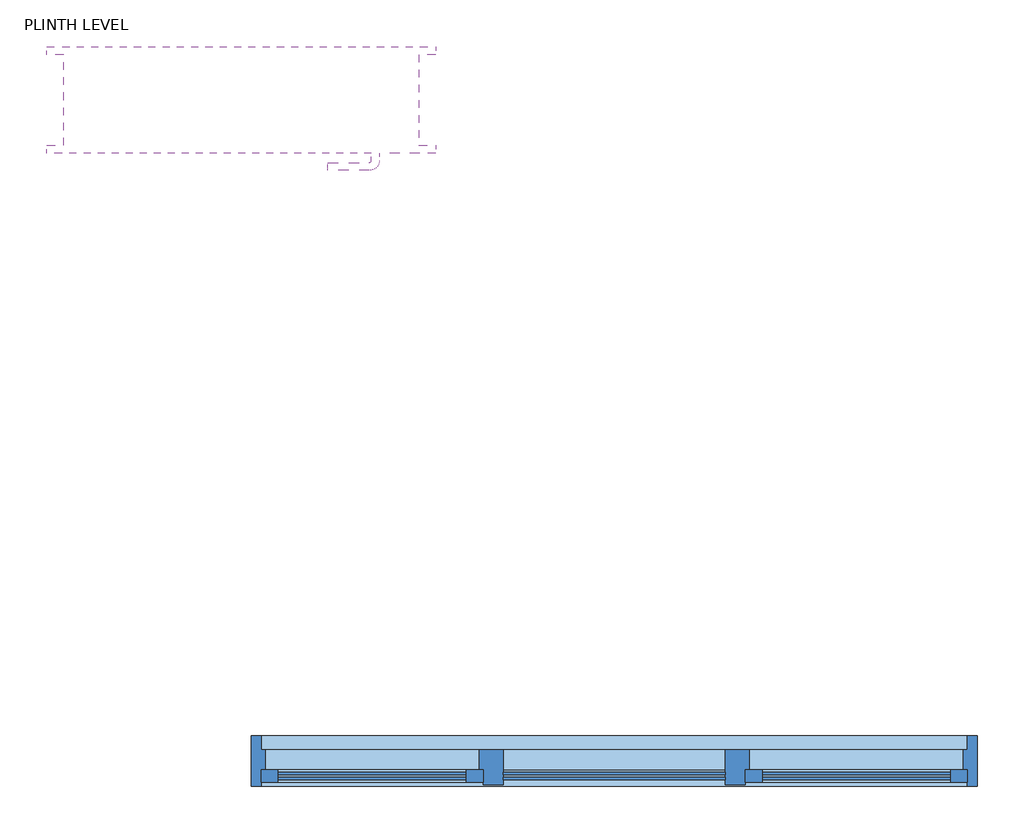
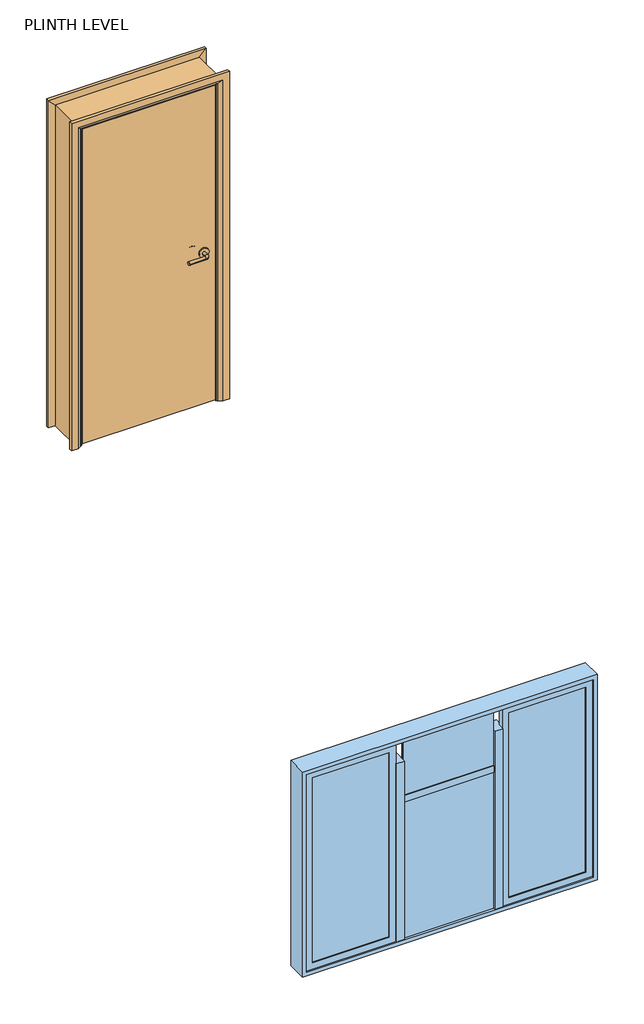
# One storey: 1 door, 1 window.
"""IFC4 building model written with IfcOpenShell, lengths in millimetres."""

from ifc_helpers import new_model, si_unit, origin, place, context, project, spatial, transform, mapped, element, save
from components import doors_intsgl_910x2110mm_6866c2a0, window_d2cb8397

model = new_model("IFC4")

# Units and contexts
model_context = context("Model", 3, world=origin())
ifc_project = project(units=[si_unit("LENGTHUNIT", "METRE", prefix="MILLI")], contexts=[model_context])

# Site, building, storey
site = spatial("IfcSite", under=ifc_project)
building = spatial("IfcBuilding", under=site)
storey = spatial("IfcBuildingStorey", under=building, Name="PLINTH LEVEL", Elevation=1371.6)

# Door
placement = place(None, origin())
doors_intsgl_910x2110mm_shape = doors_intsgl_910x2110mm_6866c2a0(model_context)
element("IfcDoor", 1, ObjectType="Doors_IntSgl : 910x2110mm", at=placement, inside=storey, context=model_context, shape_type="MappedRepresentation", body=[
    mapped(doors_intsgl_910x2110mm_shape, transform((3949.2808585, -6811.7053244, 4876.1169892), x_axis=(-1.0, 0.0, 0.0), y_axis=(0.0, -1.0, 0.0), z_axis=(0.0, 0.0, 1.0))),
])

# Window
window_shape = window_d2cb8397(model_context)
element("IfcWindow", 2, ObjectType="Window-Casement-Triple-Middle-Transom : 72\" x 53\"", at=placement, inside=storey, context=model_context, shape_type="MappedRepresentation", body=[
    mapped(window_shape, transform((4888.6722446, -8475.4053244, 1294.6178666), x_axis=(-1.0, 0.0, 0.0), y_axis=(0.0, -1.0, 0.0), z_axis=(0.0, 0.0, 1.0))),
])

save(model, "model.ifc")

# Revit data of these elements
# Type "Doors_IntSgl : 910x2110mm"
#   Construction Type Id = "MDOOR"
#   Type Mark = "41"
#   Type Comments = "Internal Single"
#   Operation = "SingleSwingRight"
#   Manufacturer = "Revit"
#   Keynote = "L20"
#   Description = "Internal Single Door"
#   Analytic Construction = "Metal"
#   UnderCut = 0' - 0.31496"
#   Tolerance = 0' - 0.07874"
#   Thickness = 0' - 1.49606"
#   Thermal Resistance (R) = 0.270117 (m²·K)/W
#   Structural Tolerance = 0' - 0.31496"
#   StopDepth = 0' - 1.25984"
#   Stop Thickness = 0' - 0.74803"
#   Rough Width = 2' - 11.82677"
#   Rough Height = 6' - 11.07087"
#   Height to Top Lock Rail = 3' - 3.37008"
#   Heat Transfer Coefficient (U) = 3.7021 W/(m²·K)
#   Handle Z Distance = 3' - 3.37008"
#   Handle X Distance = 0' - 2.95276"
#   Frame Thickness = 0' - 1.25984"
#   Door Panel Width = 2' - 8.51969"
#   Door Panel Thickness = 0' - 1.49606"
#   Door Panel Offset = 0' - 0"
#   Height = 6' - 11.07087"
#   Width = 2' - 11.82677"
#   Door Panel Height = 6' - 9.10236"
#   Architrave Setback = 0' - 0.19685"
#   Define Thermal Properties by = 1
#   Vis - Ironmongery = yes
#   Material Ironmongery = Door - Handle
#   Material Frame = Door - Frame/Mullion (1)
#   Material Door = Door - Panel
#   Material Architrave = Door - Architrave
#   Visual Light Transmittance = 0
#   Solar Heat Gain Coefficient = 0
#   Function = (empty or 0)
#   Wall Closure = (empty or 0)
# Type "Window-Casement-Triple-Middle-Transom : 72\" x 53\""
#   Type Mark = "52"
#   Fire Rating = "0.5h"
#   Assembly Code = "B2020100"
#   Analytic Construction = "Double glazing - domestic"
#   Window Width = 2' - 0"
#   Window Inset [instance default] = 0' - 0 5/8"
#   Wall Thickness [instance default] = 0' - 6"
#   Visual Light Transmittance = 0.81
#   Transom Height Ratio = 0.3
#   Thermal Resistance (R) = 0.319569 (m²·K)/W
#   Solar Heat Gain Coefficient = 0.76
#   Rough Width = 6' - 0 1/2"
#   Rough Height = 4' - 5 1/2"
#   Heat Transfer Coefficient (U) = 3.12929 W/(m²·K)
#   Height = 4' - 5"
#   Transom Height = 1' - 3.9"
#   Frame Gap 3 [instance default] = 0' - 1 83/128"
#   Frame Gap 2 [instance default] = 0' - 0 5/8"
#   Frame Gap 1 = 0' - 1 51/128"
#   Default Sill Height = 3' - 0"
#   Width = 6' - 0"
#   Frame Material = Metal - Aluminum
#   Glass Panel Material = Glass
#   Wall Closure = (empty or 0)
# Element 1 (IfcDoor, "Doors_IntSgl : 910x2110mm")
#   Phase Created = New Construction
#   Materials on its faces: "Door - Architrave", "Door - Handle", "Door - Frame/Mullion (1)", "Door - Panel"
# Element 2 (IfcWindow, "Window-Casement-Triple-Middle-Transom : 72\" x 53\"")
#   Mark = "6"
#   Window Inset = 0' - 0 5/8"
#   Frame Gap 3 = 0' - 1 83/128"
#   Frame Gap 2 = 0' - 0 5/8"
#   Phase Created = New Construction
#   Materials on its faces: "Metal - Aluminum", "Glass"
# Materials
#   "Door - Handle": colour RGB 0 0 0, transparency 0, Keynote = "P21", Cost = 0
#   "Door - Frame/Mullion (1)": class "Wood", colour RGB 212 179 113, transparency 0, Keynote = "L20", Cost = 0
#   "Door - Panel": class "Wood", colour RGB 210 159 95, transparency 0, Keynote = "L20", Cost = 0
#   "Door - Architrave": class "Wood", colour RGB 154 90 5, transparency 0, Keynote = "P20", Cost = 0
#   "Metal - Aluminum": class "Metal", colour RGB 247 247 247, transparency 0
#   "Glass": class "Glass", colour RGB 0 128 192, transparency 0.9, Description = "Soda Lime Glass", Cost = 0
